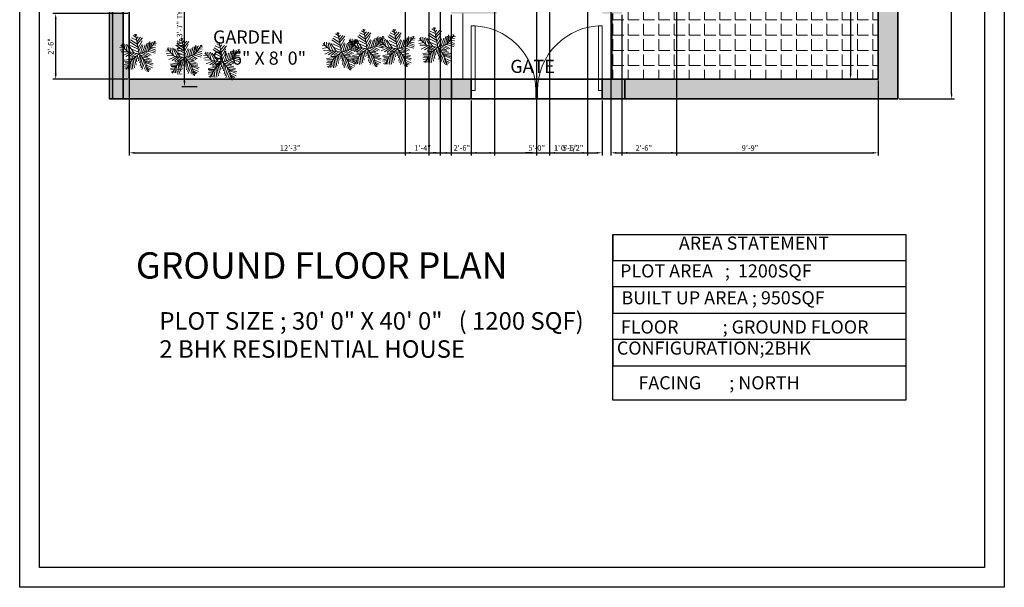
# Model space of a CAD drawing. Units: inches. Extents: x 2998 to 3448, y 1620 to 2377.
# Tile 1 of 5: x 2998 to 3448, y 1620 to 1879. Entities that reach past the tile are written whole.
import ezdxf

# ---------------------------------------------------------------- set-up
doc = ezdxf.new("R2010")
doc.units = ezdxf.units.IN
doc.layers.get('Defpoints').update_dxf_attribs({"color": 110})
for name, color, linetype, lineweight in [('A-ANNO-DIMS', 2, 'Continuous', 18), ('A-ANNO-TEXT', 7, 'Continuous', 25), ('A-ANNO-TTLB', 7, 'Continuous', 25), ('A-AREA-IDEN', 130, 'Continuous', 18), ('A-DOOR', 3, 'Continuous', 18), ('A-WALL-PATT', 18, 'Continuous', 13), ('C-PROP', 7, 'Continuous', 35), ('L-HRDS', 8, 'Continuous', 18), ('L-HRDS-PATT', 175, 'Continuous', 13), ('L-PLNT', 94, 'Continuous', 18)]:
    doc.layers.add(name, color=color, linetype=linetype, lineweight=lineweight)
doc.styles.get("Standard").update_dxf_attribs({"font": 'arial.ttf'})
doc.dimstyles.new('Copy of ISO-25', dxfattribs={"dimtxt": 2.5, "dimasz": 2.5, "dimexe": 1.25, "dimexo": 0.625, "dimtad": 1, "dimdec": 1, "dimlunit": 4, "dimtxsty": 'Standard', "dimcen": 2.5, "dimadec": 0, "dimazin": 0, "dimtfac": 1, "dimtdec": 1, "dimtmove": 0, "dimatfit": 3, "dimfxl": 1, "dimarcsym": 0})

# ---------------------------------------------------------------- blocks, each defined once
blk = doc.blocks.new('*U2')
for p, q in [((0, 0), (0, -100)), ((750, 0), (750, -100))]:
    blk.add_line(p, q)
blk.add_lwpolyline([(0, 0), (0, 750), (43.75, 750), (43.75, 0)], close=True)
blk.add_arc((0, 0), 750, 0, 90)
blk = doc.blocks.new('*U3')
for p, q in [((-750, 0), (-750, -100)), ((0, 0), (0, -100))]:
    blk.add_line(p, q)
blk.add_lwpolyline([(0, 0), (0, 750), (-43.75, 750), (-43.75, 0)], close=True)
blk.add_arc((0, 0), 750, 90, 180)
blk = doc.blocks.new('*D4')
at = {"layer": 'A-ANNO-DIMS', "color": 0, "lineweight": -2, "transparency": 16777216}
for p, q in [((3389.49, 1950.77), (3376.33, 1950.77)), ((3377.58, 1948.27), (3377.58, 1854.27)), ((3389.49, 1851.77), (3376.33, 1851.77))]:
    blk.add_line(p, q, dxfattribs=at)
at = {"layer": 'A-ANNO-DIMS', "color": 0, "transparency": 16777216}
for points in [[(3377.16, 1948.27), (3378, 1948.27), (3377.58, 1950.77)], [(3377.16, 1854.27), (3378, 1854.27), (3377.58, 1851.77)]]:
    blk.add_solid(points, dxfattribs=at)
at = {"layer": 'Defpoints', "color": 0, "transparency": 16777216}
for p in [(3390.12, 1950.77), (3377.58, 1851.77), (3390.12, 1851.77)]:
    blk.add_point(p, dxfattribs=at)
at = {"layer": 'A-ANNO-DIMS', "color": 0, "transparency": 16777216, "insert": (3375.68, 1901.27), "char_height": 2.5, "attachment_point": 5, "rotation": 90}
blk.add_mtext('8\'-3"', dxfattribs=at)
blk = doc.blocks.new('Trees - Imperial')
for p, q in [((-48.585, 21.131), (-49.309, 29.026)), ((-43.513, 28.561), (-42.427, 15.558)), ((-3.665, 19.273), (-27.574, 35.527)), ((-5.114, 28.097), (-24.676, 40.636)), ((-7.288, 39.707), (-21.778, 46.673)), ((-8.737, 47.138), (-17.069, 52.711)), ((-10.186, 53.64), (-13.084, 55.962)), ((0, 0), (-10.5, 57)), ((-9.099, 51.782), (-6.563, 55.962)), ((-7.65, 43.423), (-2.578, 49.46)), ((-5.839, 35.992), (4.667, 48.067)), ((-5.114, 27.632), (10.463, 46.673)), ((-2.941, 16.486), (8.652, 37.85)), ((16.259, 5.805), (23.142, 31.348)), ((22.055, 7.198), (27.489, 32.277)), ((27, 9), (48, 36)), ((27.127, 9.056), (31.112, 35.992)), ((31.836, 30.883), (32.561, 16.486)), ((35.096, 32.741), (37.27, 22.524)), ((38.719, 34.134), (41.979, 28.561)), ((43.791, 29.954), (51.036, 30.883)), ((44.153, 36.456), (45.239, 32.741)), ((-47.498, 19.737), (-55.83, 18.344)), ((-40.615, 13.7), (-55.105, 10.913)), ((-31.5, 4.5), (-52.5, 25.5)), ((-33.37, 6.269), (-52.207, 5.34)), ((-28.299, 3.483), (-47.86, -5.805)), ((-38.442, 26.239), (-34.819, 7.663)), ((-21.416, 3.018), (-38.079, -8.128)), ((-35.544, 28.097), (-24.314, 3.947)), ((0, 0), (-31.5, 4.5)), ((-14.533, 2.09), (-30.834, 25.31)), ((-15.982, 2.09), (-30.11, -9.521)), ((-24.314, 23.917), (-2.941, 13.7)), ((0, 0), (-22.5, -19.5)), ((-6.563, 1.161), (-21.416, -8.128)), ((-20.691, 13.7), (-1.129, 4.876)), ((-1.129, 6.734), (9.014, 26.704)), ((0, 0), (27, 9)), ((0, 0), (18, -22.5)), ((3.942, 1.625), (11.187, 24.381)), ((6.478, 1.625), (26.04, -8.592)), ((10.101, 3.483), (17.708, 26.239)), ((11.187, 3.483), (30.749, -5.805)), ((18.07, 5.805), (35.096, -3.483)), ((24.229, 7.663), (46.688, 1.625)), ((29.662, 12.307), (48.137, 6.269)), ((33.285, 16.486), (48.862, 10.913)), ((36.183, 19.737), (48.137, 17.88)), ((40.53, 25.775), (48.862, 24.846)), ((-17.431, -15.094), (-42.789, -18.809)), ((-24.314, -21.596), (-42.427, -22.06)), ((-26.849, -26.24), (-40.253, -25.775)), ((-22.5, -19.5), (-37.5, -45)), ((-15.257, -12.772), (-30.11, -12.772)), ((-25.038, -23.918), (-22.865, -45.281)), ((-20.691, -18.345), (-17.793, -44.352)), ((-6.563, -5.805), (-19.967, -9.985)), ((-17.069, -15.094), (-12.721, -40.172)), ((-13.446, -11.378), (-8.737, -32.741)), ((-9.461, -8.592), (-6.201, -23.453)), ((-4.752, -3.483), (-3.665, -14.629)), ((2.493, -3.019), (-1.491, -20.202)), ((1.769, -2.555), (24.229, -9.521)), ((5.029, -6.27), (2.131, -25.775)), ((9.014, -11.378), (3.58, -35.992)), ((14.085, -16.951), (6.478, -40.172)), ((7.565, -9.056), (32.198, -14.629)), ((18.07, -22.524), (8.289, -45.745)), ((12.274, -15.094), (36.907, -18.809)), ((16.259, -19.738), (36.183, -22.989)), ((18, -22.5), (27, -52.5)), ((18.433, -22.524), (40.53, -29.026)), ((19.157, -25.311), (38.719, -33.206)), ((-28.299, -29.026), (-42.789, -31.348)), ((-30.834, -34.135), (-42.427, -35.528)), ((-34.457, -39.708), (-40.978, -42.494)), ((-32.646, -36.921), (-31.921, -44.352)), ((-29.023, -30.884), (-27.936, -43.887)), ((20.244, -30.419), (15.897, -44.816)), ((22.78, -37.85), (19.519, -48.532)), ((21.331, -32.741), (39.081, -40.636)), ((22.78, -38.314), (34.372, -44.816)), ((24.591, -45.745), (23.142, -50.854)), ((24.591, -43.423), (30.749, -47.603)), ((26.764, -49.925), (28.213, -50.854))]:
    blk.add_line(p, q)
blk = doc.blocks.new('*D27')
at = {"layer": 'A-ANNO-DIMS', "color": 0, "lineweight": -2, "transparency": 16777216}
for p, q in [((3079.17, 1891.4), (3072.1, 1891.4)), ((3073.35, 1850.88), (3073.35, 1888.9)), ((3079.17, 1848.38), (3072.1, 1848.38))]:
    blk.add_line(p, q, dxfattribs=at)
at = {"layer": 'A-ANNO-DIMS', "color": 0, "transparency": 16777216}
for points in [[(3072.93, 1888.9), (3073.76, 1888.9), (3073.35, 1891.4)], [(3072.93, 1850.88), (3073.76, 1850.88), (3073.35, 1848.38)]]:
    blk.add_solid(points, dxfattribs=at)
at = {"layer": 'Defpoints', "color": 0}
for p in [(3073.35, 1891.4), (3079.8, 1891.4), (3079.8, 1848.38)]:
    blk.add_point(p, dxfattribs=at)
at = {"layer": 'A-ANNO-DIMS', "color": 0, "transparency": 16777216, "insert": (3071.43, 1869.89), "char_height": 2.5, "attachment_point": 5, "rotation": 90}
blk.add_mtext('PLANTING 3\'-7" TYP.', dxfattribs=at)
blk = doc.blocks.new('*D40')
at = {"layer": 'A-ANNO-DIMS', "color": 0, "lineweight": -2, "transparency": 16777216}
for p, q in [((3399.74, 2322.77), (3424.97, 2322.77)), ((3423.72, 1845.27), (3423.72, 2320.27)), ((3399.74, 1842.77), (3424.97, 1842.77))]:
    blk.add_line(p, q, dxfattribs=at)
at = {"layer": 'A-ANNO-DIMS', "color": 0, "transparency": 16777216}
for points in [[(3423.3, 2320.27), (3424.14, 2320.27), (3423.72, 2322.77)], [(3423.3, 1845.27), (3424.14, 1845.27), (3423.72, 1842.77)]]:
    blk.add_solid(points, dxfattribs=at)
at = {"layer": 'Defpoints', "color": 0}
for p in [(3399.12, 2322.77), (3423.72, 2322.77), (3399.12, 1842.77)]:
    blk.add_point(p, dxfattribs=at)
at = {"layer": 'A-ANNO-DIMS', "color": 0, "transparency": 16777216, "insert": (3421.82, 2082.77), "char_height": 2.5, "attachment_point": 5, "rotation": 90}
blk.add_mtext('40\'-0"', dxfattribs=at)
blk = doc.blocks.new('*D42')
at = {"layer": 'A-ANNO-DIMS', "color": 0, "lineweight": -2, "transparency": 16777216}
for p, q in [((3047.49, 1881.77), (3013.27, 1881.77)), ((3014.52, 1854.27), (3014.52, 1879.27)), ((3047.49, 1851.77), (3013.27, 1851.77))]:
    blk.add_line(p, q, dxfattribs=at)
at = {"layer": 'A-ANNO-DIMS', "color": 0, "transparency": 16777216}
for points in [[(3014.1, 1879.27), (3014.94, 1879.27), (3014.52, 1881.77)], [(3014.1, 1854.27), (3014.94, 1854.27), (3014.52, 1851.77)]]:
    blk.add_solid(points, dxfattribs=at)
at = {"layer": 'Defpoints', "color": 0}
for p in [(3014.52, 1881.77), (3048.12, 1881.77), (3048.12, 1851.77)]:
    blk.add_point(p, dxfattribs=at)
at = {"layer": 'A-ANNO-DIMS', "color": 0, "transparency": 16777216, "insert": (3012.62, 1866.77), "char_height": 2.5, "attachment_point": 5, "rotation": 90}
blk.add_mtext('2\'-6"', dxfattribs=at)
blk = doc.blocks.new('*D43')
at = {"layer": 'A-ANNO-DIMS', "color": 0, "lineweight": -2, "transparency": 16777216}
for p, q in [((3048.12, 1881.15), (3048.12, 1816.92)), ((3195.12, 1881.15), (3195.12, 1816.92)), ((3050.62, 1818.17), (3192.62, 1818.17))]:
    blk.add_line(p, q, dxfattribs=at)
at = {"layer": 'A-ANNO-DIMS', "color": 0, "transparency": 16777216}
for points in [[(3050.62, 1818.59), (3050.62, 1817.76), (3048.12, 1818.17)], [(3192.62, 1818.59), (3192.62, 1817.76), (3195.12, 1818.17)]]:
    blk.add_solid(points, dxfattribs=at)
at = {"layer": 'Defpoints', "color": 0}
for p in [(3048.12, 1881.77), (3195.12, 1881.77), (3195.12, 1818.17)]:
    blk.add_point(p, dxfattribs=at)
at = {"layer": 'A-ANNO-DIMS', "color": 0, "transparency": 16777216, "insert": (3121.62, 1820.07), "char_height": 2.5, "attachment_point": 5}
blk.add_mtext('12\'-3"', dxfattribs=at)
blk = doc.blocks.new('*D44')
at = {"layer": 'A-ANNO-DIMS', "color": 0, "lineweight": -2, "transparency": 16777216}
for p, q in [((3204.35, 1842.15), (3204.35, 1816.92)), ((3264.12, 1842.15), (3264.12, 1816.92)), ((3206.85, 1818.17), (3261.62, 1818.17))]:
    blk.add_line(p, q, dxfattribs=at)
at = {"layer": 'A-ANNO-DIMS', "color": 0, "transparency": 16777216}
for points in [[(3206.85, 1818.59), (3206.85, 1817.76), (3204.35, 1818.17)], [(3261.62, 1818.59), (3261.62, 1817.76), (3264.12, 1818.17)]]:
    blk.add_solid(points, dxfattribs=at)
at = {"layer": 'Defpoints', "color": 0}
for p in [(3204.35, 1842.77), (3264.12, 1842.77), (3264.12, 1818.17)]:
    blk.add_point(p, dxfattribs=at)
at = {"layer": 'A-ANNO-DIMS', "color": 0, "transparency": 16777216, "insert": (3234.23, 1820.07), "char_height": 2.5, "attachment_point": 5}
blk.add_mtext('5\'-0"', dxfattribs=at)
blk = doc.blocks.new('*D45')
at = {"layer": 'A-ANNO-DIMS', "color": 0, "lineweight": -2, "transparency": 16777216}
for p, q in [((3273.12, 1881.15), (3273.12, 1816.92)), ((3390.12, 1851.15), (3390.12, 1816.92)), ((3275.62, 1818.17), (3387.62, 1818.17))]:
    blk.add_line(p, q, dxfattribs=at)
at = {"layer": 'A-ANNO-DIMS', "color": 0, "transparency": 16777216}
for points in [[(3275.62, 1818.59), (3275.62, 1817.76), (3273.12, 1818.17)], [(3387.62, 1818.59), (3387.62, 1817.76), (3390.12, 1818.17)]]:
    blk.add_solid(points, dxfattribs=at)
at = {"layer": 'Defpoints', "color": 0}
for p in [(3273.12, 1881.77), (3390.12, 1851.77), (3390.12, 1818.17)]:
    blk.add_point(p, dxfattribs=at)
at = {"layer": 'A-ANNO-DIMS', "color": 0, "transparency": 16777216, "insert": (3331.62, 1820.07), "char_height": 2.5, "attachment_point": 5}
blk.add_mtext('9\'-9"', dxfattribs=at)
blk = doc.blocks.new('*D51')
at = {"layer": 'A-ANNO-DIMS', "color": 0, "lineweight": -2, "transparency": 16777216}
for p, q in [((3174.12, 2256.15), (3174.12, 1816.92)), ((3190.13, 2256.15), (3190.13, 1816.92)), ((3176.62, 1818.17), (3187.63, 1818.17))]:
    blk.add_line(p, q, dxfattribs=at)
at = {"layer": 'A-ANNO-DIMS', "color": 0, "transparency": 16777216}
for points in [[(3176.62, 1818.59), (3176.62, 1817.76), (3174.12, 1818.17)], [(3187.63, 1818.59), (3187.63, 1817.76), (3190.13, 1818.17)]]:
    blk.add_solid(points, dxfattribs=at)
at = {"layer": 'Defpoints', "color": 0}
for p in [(3174.12, 2256.77), (3190.13, 2256.77), (3190.13, 1818.17)]:
    blk.add_point(p, dxfattribs=at)
at = {"layer": 'A-ANNO-DIMS', "color": 0, "transparency": 16777216, "insert": (3182.12, 1820.05), "char_height": 2.5, "attachment_point": 5}
blk.add_mtext('1\'-4"', dxfattribs=at)
blk = doc.blocks.new('*D52')
at = {"layer": 'A-ANNO-DIMS', "color": 0, "lineweight": -2, "transparency": 16777216}
for p, q in [((3240.12, 2256.15), (3240.12, 1816.92)), ((3257.48, 2256.15), (3257.48, 1816.92)), ((3242.62, 1818.17), (3254.98, 1818.17))]:
    blk.add_line(p, q, dxfattribs=at)
at = {"layer": 'A-ANNO-DIMS', "color": 0, "transparency": 16777216}
for points in [[(3242.62, 1818.59), (3242.62, 1817.76), (3240.12, 1818.17)], [(3254.98, 1818.59), (3254.98, 1817.76), (3257.48, 1818.17)]]:
    blk.add_solid(points, dxfattribs=at)
at = {"layer": 'Defpoints', "color": 0}
for p in [(3240.12, 2256.77), (3257.48, 2256.77), (3257.48, 1818.17)]:
    blk.add_point(p, dxfattribs=at)
at = {"layer": 'A-ANNO-DIMS', "color": 0, "transparency": 16777216, "insert": (3248.8, 1820.09), "char_height": 2.5, "attachment_point": 5}
blk.add_mtext('1\'-5 1/2"', dxfattribs=at)
blk = doc.blocks.new('*D54')
at = {"layer": 'A-ANNO-DIMS', "color": 0, "lineweight": -2, "transparency": 16777216}
for p, q in [((3185.01, 2154.15), (3185.01, 1816.92)), ((3215.01, 2154.15), (3215.01, 1816.92)), ((3187.51, 1818.17), (3212.51, 1818.17))]:
    blk.add_line(p, q, dxfattribs=at)
at = {"layer": 'A-ANNO-DIMS', "color": 0, "transparency": 16777216}
for points in [[(3187.51, 1818.59), (3187.51, 1817.76), (3185.01, 1818.17)], [(3212.51, 1818.59), (3212.51, 1817.76), (3215.01, 1818.17)]]:
    blk.add_solid(points, dxfattribs=at)
at = {"layer": 'Defpoints', "color": 0}
for p in [(3185.01, 2154.77), (3215.01, 2154.77), (3215.01, 1818.17)]:
    blk.add_point(p, dxfattribs=at)
at = {"layer": 'A-ANNO-DIMS', "color": 0, "transparency": 16777216, "insert": (3200.01, 1820.07), "char_height": 2.5, "attachment_point": 5}
blk.add_mtext('2\'-6"', dxfattribs=at)
blk = doc.blocks.new('*D55')
at = {"layer": 'A-ANNO-DIMS', "color": 0, "lineweight": -2, "transparency": 16777216}
for p, q in [((3268.12, 2154.15), (3268.12, 1816.92)), ((3298.12, 2154.15), (3298.12, 1816.92)), ((3270.62, 1818.17), (3295.62, 1818.17))]:
    blk.add_line(p, q, dxfattribs=at)
at = {"layer": 'A-ANNO-DIMS', "color": 0, "transparency": 16777216}
for points in [[(3270.62, 1818.59), (3270.62, 1817.76), (3268.12, 1818.17)], [(3295.62, 1818.59), (3295.62, 1817.76), (3298.12, 1818.17)]]:
    blk.add_solid(points, dxfattribs=at)
at = {"layer": 'Defpoints', "color": 0}
for p in [(3268.12, 2154.77), (3298.12, 2154.77), (3298.12, 1818.17)]:
    blk.add_point(p, dxfattribs=at)
at = {"layer": 'A-ANNO-DIMS', "color": 0, "transparency": 16777216, "insert": (3283.12, 1820.07), "char_height": 2.5, "attachment_point": 5}
blk.add_mtext('2\'-6"', dxfattribs=at)
blk = doc.blocks.new('*D67')
at = {"layer": 'A-ANNO-DIMS', "color": 0, "lineweight": -2, "transparency": 16777216}
for p, q in [((3234.12, 2160.15), (3234.12, 1816.92)), ((3240.12, 2160.15), (3240.12, 1816.92)), ((3231.62, 1818.17), (3229.12, 1818.17)), ((3234.12, 1818.17), (3240.12, 1818.17)), ((3242.62, 1818.17), (3253.01, 1818.17))]:
    blk.add_line(p, q, dxfattribs=at)
at = {"layer": 'A-ANNO-DIMS', "color": 0, "transparency": 16777216}
for points in [[(3231.62, 1818.59), (3231.62, 1817.76), (3234.12, 1818.17)], [(3242.62, 1818.59), (3242.62, 1817.76), (3240.12, 1818.17)]]:
    blk.add_solid(points, dxfattribs=at)
at = {"layer": 'Defpoints', "color": 0}
for p in [(3234.12, 2160.77), (3240.12, 2160.77), (3240.12, 1818.17)]:
    blk.add_point(p, dxfattribs=at)
at = {"layer": 'A-ANNO-DIMS', "color": 0, "transparency": 16777216, "insert": (3249.07, 1820.07), "char_height": 2.5, "attachment_point": 5}
blk.add_mtext('0\'-6"', dxfattribs=at)

msp = doc.modelspace()

# ---------------------------------------------------------------- hatches: boundary and pattern name
at = {"layer": 'A-WALL-PATT'}
h = msp.add_hatch(color=256, dxfattribs=at)
h.dxf.hatch_style = 1
h.paths.add_polyline_path([(3399.12, 2322.77), (3039.12, 2322.77), (3039.12, 2132.57), (3048.12, 2132.57), (3048.12, 2154.77), (3048.12, 2313.77), (3390.12, 2313.77), (3390.12, 2227.86), (3399.12, 2227.86)])
h.paths.add_polyline_path([(3048.12, 2072.57), (3039.12, 2072.57), (3039.12, 2041.4), (3048.12, 2041.4)])
h.paths.add_polyline_path([(3399.12, 1997.2), (3390.12, 1997.2), (3390.12, 1851.77), (3274.41, 1851.77), (3274.41, 1842.77), (3399.12, 1842.77)])
h.paths.add_polyline_path([(3195.35, 1851.77), (3048.12, 1851.77), (3048.12, 1857.27), (3048.05, 1858.06), (3047.68, 1858.02), (3047.44, 1857.61), (3047.47, 1857.28), (3047.17, 1857.15), (3047.68, 1858.02), (3045.29, 1857.73), (3045.29, 1842.77), (3195.35, 1842.77)])
h.paths.add_polyline_path([(3399.12, 2167.86), (3390.12, 2167.86), (3390.12, 2112.77), (3390.12, 2103.77), (3390.12, 2045.2), (3399.12, 2045.2)])
h.paths.add_polyline_path([(3390.12, 2112.77), (3306.12, 2112.77), (3306.12, 2118.77), (3304.88, 2118.77), (3300.12, 2118.77), (3300.12, 2112.77), (3300.12, 2103.77), (3390.12, 2103.77)])
h.paths.add_polyline_path([(3257.48, 2265.77), (3214.13, 2265.77), (3214.13, 2256.77), (3257.48, 2256.77)], flags=17)
h.paths.add_polyline_path([(3325.36, 2265.77), (3281.48, 2265.77), (3281.48, 2256.77), (3300.12, 2256.77), (3325.36, 2256.77)], flags=17)
h.paths.add_polyline_path([(3390.12, 2265.77), (3373.36, 2265.77), (3373.36, 2256.77), (3390.12, 2256.77)], flags=17)
h.paths.add_polyline_path([(3190.13, 2265.77), (3155.91, 2265.77), (3155.91, 2256.77), (3190.13, 2256.77)], flags=17)
h.paths.add_polyline_path([(3306.12, 2256.77), (3300.12, 2256.77), (3300.12, 2160.77), (3298.12, 2160.77), (3298.12, 2154.77), (3300.12, 2154.77), (3306.12, 2154.77)], flags=17)
h.paths.add_polyline_path([(3240.12, 2256.77), (3234.12, 2256.77), (3234.12, 2160.77), (3215.01, 2160.77), (3215.01, 2154.77), (3268.12, 2154.77), (3268.12, 2158.71), (3268.12, 2160.77), (3240.12, 2160.77)], flags=17)
h.paths.add_polyline_path([(3174.12, 2256.77), (3168.12, 2256.77), (3168.12, 2160.77), (3138.26, 2160.77), (3138.26, 2154.77), (3174.12, 2154.77), (3185.01, 2154.77), (3185.01, 2158.71), (3185.01, 2160.77), (3174.12, 2160.77)], flags=17)
h.paths.add_polyline_path([(3090.26, 2160.77), (3048.12, 2160.77), (3048.12, 2154.77), (3090.26, 2154.77)], flags=17)
h.paths.add_polyline_path([(3072.12, 2058.77), (3048.12, 2058.77), (3048.12, 2049.77), (3072.12, 2049.77)])
h.paths.add_polyline_path([(3298.3, 1959.77), (3270.12, 1959.77), (3270.12, 2061.77), (3300.12, 2061.77), (3306.12, 2061.77), (3306.12, 2067.77), (3300.12, 2067.77), (3264.12, 2067.77), (3264.12, 2061.77), (3264.12, 1959.77), (3252.12, 1959.77), (3252.12, 1955.56), (3252.12, 1950.77), (3264.12, 1950.77), (3264.12, 1890.77), (3264.12, 1881.77), (3273.12, 1881.77), (3273.12, 1950.77), (3298.3, 1950.77)])
h.paths.add_polyline_path([(3390.12, 1959.77), (3358.3, 1959.77), (3358.3, 1950.77), (3390.12, 1950.77)], flags=17)
h.paths.add_polyline_path([(3216.12, 1959.77), (3154.02, 1959.77), (3154.02, 1950.77), (3216.12, 1950.77)])
h.paths.add_polyline_path([(3204.12, 1950.77), (3195.12, 1950.77), (3195.12, 1890.77), (3195.12, 1881.77), (3216.12, 1881.77), (3216.12, 1890.77), (3204.12, 1890.77)])
h.paths.add_polyline_path([(3094.02, 1959.77), (3048.12, 1959.77), (3048.12, 1950.77), (3094.02, 1950.77)])
h.paths.add_polyline_path([(3045.29, 1981.4), (3040.45, 1981.4), (3040.45, 1842.77), (3045.29, 1842.77), (3045.29, 1857.73)])
h.paths.add_polyline_path([(3059.91, 2261.45), (3059.91, 2265.77), (3048.12, 2265.77), (3048.12, 2256.77), (3059.91, 2256.77)], flags=17)
h.paths.add_polyline_path([(3107.91, 2265.77), (3095.91, 2265.77), (3095.91, 2256.77), (3107.91, 2256.77)], flags=17)
h.paths.add_polyline_path([(3274.41, 1851.77), (3264.12, 1851.77), (3264.12, 1846.71), (3264.12, 1842.77), (3274.41, 1842.77)])
h.paths.add_polyline_path([(3204.35, 1851.77), (3195.35, 1851.77), (3195.35, 1842.77), (3204.35, 1842.77), (3204.35, 1846.71)])
at = {"layer": 'L-HRDS-PATT'}
h = msp.add_hatch(dxfattribs=at)
h.set_pattern_fill('ANGLE', color=256)
h.set_pattern_definition([(0, (0, 0), (0, 6.985), [5.08, -1.905]), (90, (0, 0), (-6.985, 4e-16), [5.08, -1.905])])
h.paths.add_polyline_path([(3390.12, 1950.77), (3358.3, 1950.77), (3273.12, 1950.77), (3273.12, 1881.77), (3268.62, 1881.77), (3268.62, 1851.77), (3390.12, 1851.77)])
h.paths.add_polyline_path([(3334.58, 2144.47), (3389.67, 2144.47), (3389.67, 2153.66), (3334.58, 2153.66)], flags=9)
h.paths.add_polyline_path([(3334.56, 2154.09), (3390.29, 2154.09), (3390.29, 2163.4), (3334.56, 2163.4)], flags=9)
h.paths.add_polyline_path([(3220.44, 1918.61), (3261.55, 1918.61), (3261.55, 1927.8), (3220.44, 1927.8)], flags=9)
h.paths.add_polyline_path([(3220.42, 1928.23), (3252.4, 1928.23), (3252.4, 1937.54), (3220.42, 1937.54)], flags=9)
h.paths.add_polyline_path([(3220.62, 1853.01), (3246.55, 1853.01), (3246.55, 1862.32), (3220.62, 1862.32)], flags=9)
h.paths.add_polyline_path([(3084.85, 1856.81), (3130.62, 1856.81), (3130.62, 1866), (3084.85, 1866)], flags=9)
h.paths.add_polyline_path([(3084.83, 1866.42), (3123.8, 1866.42), (3123.8, 1875.73), (3084.83, 1875.73)], flags=9)
h.paths.add_polyline_path([(3297.1, 1896.73), (3349.87, 1896.73), (3349.87, 1905.92), (3297.1, 1905.92)], flags=24)
h.paths.add_polyline_path([(3297.08, 1906.35), (3357.94, 1906.35), (3357.94, 1915.66), (3297.08, 1915.66)], flags=24)
h.paths.add_polyline_path([(3107.62, 2003.86), (3160.38, 2003.86), (3160.38, 2013.05), (3107.62, 2013.05)], flags=9)
h.paths.add_polyline_path([(3107.6, 2013.48), (3161.48, 2013.48), (3161.48, 2022.79), (3107.6, 2022.79)], flags=9)
h.paths.add_polyline_path([(3294.47, 2015.87), (3347.23, 2015.87), (3347.23, 2025.06), (3294.47, 2025.06)], flags=9)
h.paths.add_polyline_path([(3294.45, 2025.49), (3350.19, 2025.49), (3350.19, 2034.8), (3294.45, 2034.8)], flags=9)
h.paths.add_polyline_path([(3162.21, 2109.19), (3212.64, 2109.19), (3212.64, 2118.38), (3162.21, 2118.38)], flags=9)
h.paths.add_polyline_path([(3162.19, 2118.81), (3194.63, 2118.81), (3194.63, 2128.12), (3162.19, 2128.12)], flags=9)
h.paths.add_polyline_path([(3075.92, 2206.31), (3126.35, 2206.31), (3126.35, 2215.5), (3075.92, 2215.5)], flags=9)
h.paths.add_polyline_path([(3075.9, 2215.93), (3115.79, 2215.93), (3115.79, 2225.24), (3075.9, 2225.24)], flags=9)

# ---------------------------------------------------------------- linework, layer by layer
at = {"layer": 'A-ANNO-TTLB'}
for p, q in [((3268.94, 1780.91), (3268.94, 1768.91)), ((3268.94, 1768.91), (3402.77, 1768.91)), ((3402.77, 1768.91), (3402.77, 1756.91)), ((3402.77, 1756.91), (3268.94, 1756.91)), ((3268.94, 1756.91), (3268.94, 1744.91)), ((3268.94, 1744.91), (3402.77, 1744.91)), ((3402.77, 1744.91), (3402.77, 1732.91)), ((3402.77, 1732.91), (3268.94, 1732.91)), ((3268.94, 1732.91), (3268.94, 1720.91)), ((3268.94, 1720.91), (3402.77, 1720.91))]:
    msp.add_line(p, q, dxfattribs=at)
for points in [[(2998.07, 2376.74), (3447.79, 2376.74), (3447.79, 1619.66), (2998.07, 1619.66)], [(3007.07, 2367.74), (3438.79, 2367.74), (3438.79, 1628.66), (3007.07, 1628.66)], [(3268.94, 1780.91), (3402.77, 1780.91), (3402.77, 1705.21), (3268.94, 1705.21)]]:
    msp.add_lwpolyline(points, close=True, dxfattribs=at)
at = {"layer": 'C-PROP'}
for p, q in [((3040.45, 1981.4), (3040.45, 1842.77)), ((3045.29, 1842.77), (3045.29, 1981.4)), ((3048.12, 1851.77), (3195.35, 1851.77)), ((3195.35, 1851.77), (3195.35, 1842.77)), ((3204.35, 1842.77), (3204.35, 1851.77)), ((3204.35, 1851.77), (3261.18, 1851.77)), ((3274.41, 1851.77), (3261.18, 1851.77)), ((3264.12, 1851.77), (3264.12, 1842.77)), ((3274.41, 1842.77), (3274.41, 1851.77)), ((3040.45, 1842.77), (3045.29, 1842.77)), ((3195.35, 1842.77), (3204.35, 1842.77)), ((3261.18, 1842.77), (3274.41, 1842.77))]:
    msp.add_line(p, q, dxfattribs=at)
for points in [[(3039.12, 2322.77), (3399.12, 2322.77), (3399.12, 1842.77), (3039.12, 1842.77)], [(3048.12, 2313.77), (3390.12, 2313.77), (3390.12, 1851.77), (3048.12, 1851.77)]]:
    msp.add_lwpolyline(points, close=True, dxfattribs=at)
at = {"layer": 'L-HRDS'}
for p, q in [((3200.55, 1881.77), (3200.55, 1851.77)), ((3268.62, 1881.77), (3268.62, 1851.77))]:
    msp.add_line(p, q, dxfattribs=at)

# ---------------------------------------------------------------- block references
at = {"layer": 'A-DOOR', "xscale": 0.0393700787401575, "yscale": 0.0393700787401575, "zscale": 0.0393700787401575}
for name, p in [('*U2', (3204.35, 1846.71)), ('*U3', (3264.12, 1846.71))]:
    msp.add_blockref(name, p, dxfattribs=at)
at = {"layer": 'L-PLNT', "xscale": 0.1575732095692182, "yscale": 0.1575732095692182, "zscale": 0.1575732095692182}
for p in [(3189.02, 1866.45), (3052.59, 1863.4), (3145, 1864.16), (3156.83, 1865.68), (3170.69, 1865.67), (3170.69, 1865.67), (3073.66, 1861.69), (3090.85, 1859.71)]:
    msp.add_blockref('Trees - Imperial', p, dxfattribs=at)

# ---------------------------------------------------------------- texts
at = {"layer": 'A-ANNO-TEXT'}
for s, height, p in [('AREA STATEMENT', 6, (3299.16, 1773.91)), ('GROUND FLOOR PLAN', 12, (3051.15, 1760.72)), ('PLOT AREA   ;  1200SQF', 6, (3272.28, 1761.23)), ('BUILT UP AREA ; 950SQF', 6, (3272.93, 1748.95)), ('PLOT SIZE ; 30\' 0" X 40\' 0"   ( 1200 SQF)', 8, (3061.88, 1737.38)), (' FLOOR           ; GROUND FLOOR', 6, (3270.83, 1735.61)), ('2 BHK RESIDENTIAL HOUSE', 8, (3061.88, 1724.53)), ('CONFIGURATION;2BHK', 6, (3270.83, 1725.97)), ('FACING       ; NORTH', 6, (3280.67, 1710.11))]:
    msp.add_text(s, height=height, dxfattribs=at).set_placement(p)
at = {"layer": 'A-AREA-IDEN'}
for s, p in [('GARDEN', (3086.39, 1868.08)), ('9\' 6" X 8\' 0"', (3086.39, 1858.44)), ('GATE', (3222.17, 1854.67))]:
    msp.add_text(s, height=6, dxfattribs=at).set_placement(p)

# ---------------------------------------------------------------- dimensions: what is measured, and where the dimension line sits
at = {"layer": 'A-ANNO-DIMS'}
for base, p1, p2, override, picture, middle in [((3423.72, 2322.77), (3399.12, 1842.77), (3399.12, 2322.77), {"dimdec": 1, "dimlfac": 1, "dimrnd": 0, "dimzin": 1, "dimdsep": 46, "dimlunit": 4, "dimfrac": 2}, '*D40', (3421.82, 2082.77)), ((3377.58, 1851.77), (3390.12, 1950.77), (3390.12, 1851.77), {"dimclrd": 0, "dimclre": 0, "dimclrt": 0}, '*D4', (3375.68, 1901.27)), ((3014.52, 1881.77), (3048.12, 1851.77), (3048.12, 1881.77), {"dimdec": 1, "dimlfac": 1, "dimrnd": 0, "dimzin": 1, "dimdsep": 46, "dimlunit": 4, "dimfrac": 2}, '*D42', (3012.62, 1866.77))]:
    dim = msp.add_linear_dim(base=base, p1=p1, p2=p2, angle=90, dimstyle='Copy of ISO-25', override=override, dxfattribs=at)
    dim.commit()
    dim.dimension.update_dxf_attribs({"geometry": picture, "text_midpoint": middle})
for base, p1, p2, picture, middle in [((3190.13, 1818.17), (3174.12, 2256.77), (3190.13, 2256.77), '*D51', (3182.12, 1820.05)), ((3257.48, 1818.17), (3240.12, 2256.77), (3257.48, 2256.77), '*D52', (3248.8, 1820.09)), ((3240.12, 1818.17), (3234.12, 2160.77), (3240.12, 2160.77), '*D67', (3249.07, 1820.07)), ((3215.01, 1818.17), (3185.01, 2154.77), (3215.01, 2154.77), '*D54', (3200.01, 1820.07)), ((3298.12, 1818.17), (3268.12, 2154.77), (3298.12, 2154.77), '*D55', (3283.12, 1820.07)), ((3195.12, 1818.17), (3048.12, 1881.77), (3195.12, 1881.77), '*D43', (3121.62, 1820.07)), ((3390.12, 1818.17), (3273.12, 1881.77), (3390.12, 1851.77), '*D45', (3331.62, 1820.07)), ((3264.12, 1818.17), (3204.35, 1842.77), (3264.12, 1842.77), '*D44', (3234.23, 1820.07))]:
    dim = msp.add_linear_dim(base=base, p1=p1, p2=p2, dimstyle='Copy of ISO-25', override={"dimdec": 1, "dimlfac": 1, "dimrnd": 0, "dimzin": 1, "dimdsep": 46, "dimlunit": 4, "dimfrac": 2}, dxfattribs=at)
    dim.commit()
    dim.dimension.update_dxf_attribs({"geometry": picture, "text_midpoint": middle})
dim = msp.add_linear_dim(base=(3073.35, 1891.4), p1=(3079.8, 1848.38), p2=(3079.8, 1891.4), angle=90, text='PLANTING <> TYP.', dimstyle='Copy of ISO-25', override={"dimdec": 1, "dimlfac": 1, "dimrnd": 0, "dimzin": 1, "dimdsep": 46, "dimlunit": 4, "dimfrac": 2}, dxfattribs=at)
dim.commit()
dim.dimension.update_dxf_attribs({"geometry": '*D27', "text_midpoint": (3071.43, 1869.89)})

doc.saveas('drawing.dxf')
